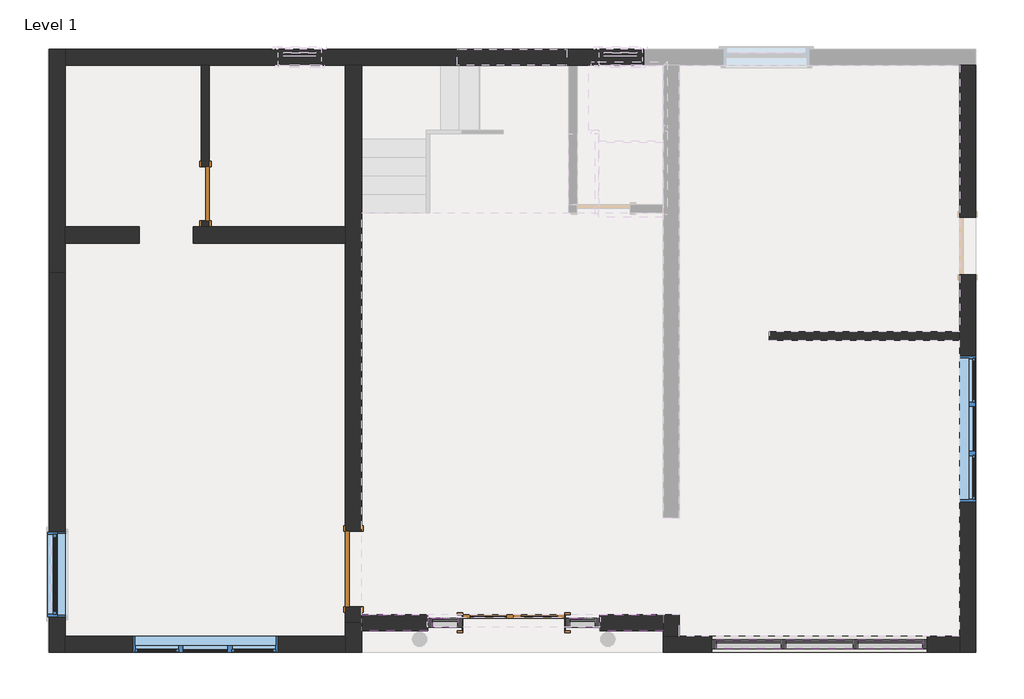
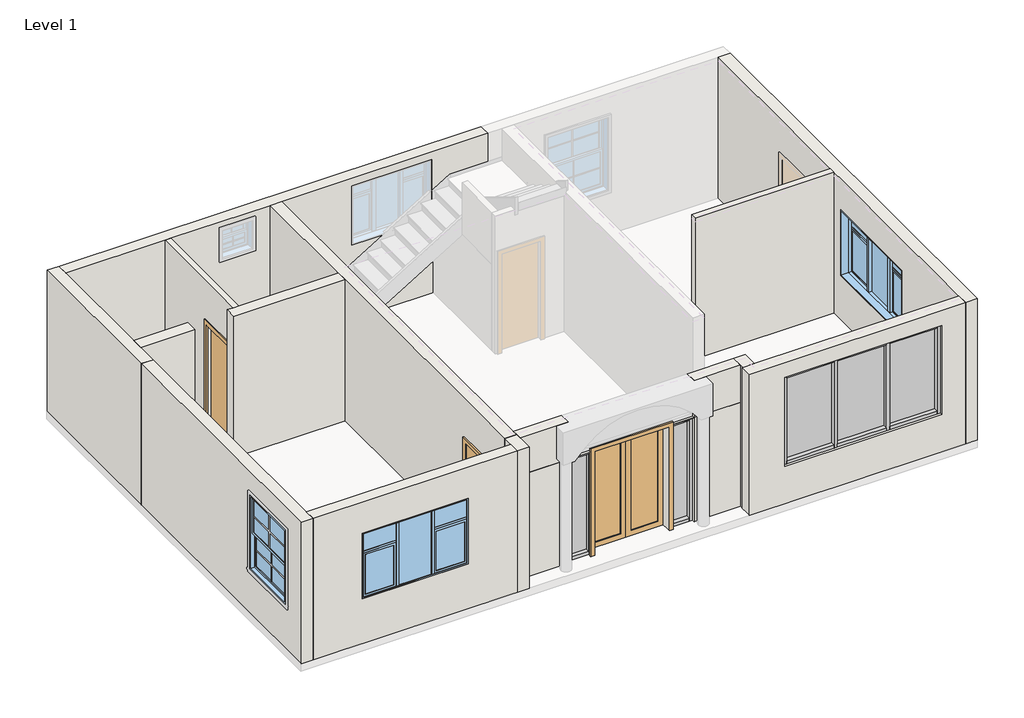
# One storey, part 1 of 2: 18 members, 16 walls, 5 plates, 3 doors, 3 windows.
"""IFC4 building model written with IfcOpenShell, lengths in millimetres."""

from ifc_helpers import new_model, si_unit, frame, origin, origin_with_axes, place, context, project, spatial, polyline, outline, extrude, faceted_brep, transform, mapped, element, save
from components import door_7b3e5dee, door_f6232a3f, door_d8f5dbb5, member_0417a2a7, member_3a4673bc, member_a7b41546, member_5da52246, member_04c9b82a, member_d60e8053, member_2fae0574, system_panel_glazed_7d1c9128, system_panel_glazed_4f997f60, system_panel_glazed_2247c2a6, system_panel_glazed_0f092676, window_casement_triple_side_transom_6_9_71562f8e, window_double_hung_3_11_b20011b0

model = new_model("IFC4")

# Units and contexts
model_context = context("Model", 3, world=origin())
ifc_project = project(units=[si_unit("LENGTHUNIT", "METRE", prefix="MILLI")], contexts=[model_context])

# Site, building, storey
site = spatial("IfcSite", under=ifc_project)
building = spatial("IfcBuilding", under=site)
storey = spatial("IfcBuildingStorey", under=building, Name="Level 1", Elevation=0.0)

# Doors
placement = place(None, origin())
door_shape = door_7b3e5dee(model_context)
element("IfcDoor", 1, ObjectType="Door-Double-Glass : 4'9\"x7'", at=placement, inside=storey, context=model_context, shape_type="MappedRepresentation", body=[
    mapped(door_shape, transform((-12852.2526022, 3914.7357665, 0.0), x_axis=(1.0, 0.0, 0.0), y_axis=(0.0, 1.0, 0.0), z_axis=(0.0, 0.0, 1.0))),
])
door_2_shape = door_f6232a3f(model_context)
element("IfcDoor", 2, ObjectType="Single-Flush : 3'6\"", at=placement, inside=storey, context=model_context, shape_type="MappedRepresentation", body=[
    mapped(door_2_shape, transform((-15119.0556236, 4679.1170165, 0.0), x_axis=(0.0, -1.0, 0.0), y_axis=(1.0, 0.0, 0.0), z_axis=(0.0, 0.0, 1.0))),
])
door_3_shape = door_d8f5dbb5(model_context)
element("IfcDoor", 3, ObjectType="Single-Flush : 30\" x 80\"", at=placement, inside=storey, context=model_context, shape_type="MappedRepresentation", body=[
    mapped(door_3_shape, transform((-17215.2240665, 9988.7207935, 0.0), x_axis=(0.0, -1.0, 0.0), y_axis=(1.0, 0.0, 0.0), z_axis=(0.0, 0.0, 1.0))),
])

# Members
member_shape = member_0417a2a7(model_context)
element("IfcMember", 4, ObjectType="Rectangular Mullion : 2.5\" x 5\" rectangular", at=placement, inside=storey, context=model_context, shape_type="MappedRepresentation", body=[
    mapped(member_shape, transform((-13645.6697078, 3917.1170165, 2128.2825), x_axis=(0.0, 0.0, 1.0), y_axis=(0.0, -1.0, 0.0), z_axis=(1.0, 0.0, 0.0))),
])
element("IfcMember", 5, ObjectType="Rectangular Mullion : 2.5\" x 5\" rectangular", at=placement, inside=storey, context=model_context, shape_type="MappedRepresentation", body=[
    mapped(member_shape, transform((-11697.1590017, 3917.1170165, 2130.0999183), x_axis=(0.0, 0.0, 1.0), y_axis=(0.0, -1.0, 0.0), z_axis=(1.0, 0.0, 0.0))),
])
element("IfcMember", 6, ObjectType="Rectangular Mullion : 2.5\" x 5\" rectangular", at=placement, inside=storey, context=model_context, shape_type="MappedRepresentation", body=[
    mapped(member_shape, transform((-14008.2736637, 3917.1170165, 0.0), x_axis=(0.0, 0.0, -1.0), y_axis=(0.0, -1.0, 0.0), z_axis=(-1.0, 0.0, 0.0))),
])
element("IfcMember", 7, ObjectType="Rectangular Mullion : 2.5\" x 5\" rectangular", at=placement, inside=storey, context=model_context, shape_type="MappedRepresentation", body=[
    mapped(member_shape, transform((-12059.7629576, 3917.1170165, 0.0), x_axis=(0.0, 0.0, -1.0), y_axis=(0.0, -1.0, 0.0), z_axis=(-1.0, 0.0, 0.0))),
])
member_2_shape = member_3a4673bc(model_context)
element("IfcMember", 8, ObjectType="Rectangular Mullion : 2.5\" x 5\" rectangular", at=placement, inside=storey, context=model_context, shape_type="MappedRepresentation", body=[
    mapped(member_2_shape, transform((-13582.1697078, 3917.1170165, 0.0), x_axis=(1.0, 0.0, 0.0), y_axis=(0.0, -1.0, 0.0), z_axis=(0.0, 0.0, -1.0))),
])
element("IfcMember", 9, ObjectType="Rectangular Mullion : 2.5\" x 5\" rectangular", at=placement, inside=storey, context=model_context, shape_type="MappedRepresentation", body=[
    mapped(member_2_shape, transform((-14071.7736637, 3917.1170165, 2128.2825), x_axis=(-1.0, 0.0, 0.0), y_axis=(0.0, -1.0, 0.0), z_axis=(0.0, 0.0, 1.0))),
])
member_3_shape = member_a7b41546(model_context)
element("IfcMember", 10, ObjectType="Rectangular Mullion : 2.5\" x 5\" rectangular", at=placement, inside=storey, context=model_context, shape_type="MappedRepresentation", body=[
    mapped(member_3_shape, transform((-11633.6590017, 3917.1170165, 0.0), x_axis=(1.0, 0.0, 0.0), y_axis=(0.0, -1.0, 0.0), z_axis=(0.0, 0.0, -1.0))),
])
element("IfcMember", 11, ObjectType="Rectangular Mullion : 2.5\" x 5\" rectangular", at=placement, inside=storey, context=model_context, shape_type="MappedRepresentation", body=[
    mapped(member_3_shape, transform((-12123.2629576, 3917.1170165, 2130.0999183), x_axis=(-1.0, 0.0, 0.0), y_axis=(0.0, -1.0, 0.0), z_axis=(0.0, 0.0, 1.0))),
])
member_4_shape = member_5da52246(model_context)
element("IfcMember", 12, ObjectType="Rectangular Mullion : 2.5\" x 5\" rectangular", at=placement, inside=storey, context=model_context, shape_type="MappedRepresentation", body=[
    mapped(member_4_shape, transform((-7064.7325804, 3612.4962903, 2590.8), x_axis=(0.0, 0.0, 1.0), y_axis=(0.0, -1.0, 0.0), z_axis=(1.0, 0.0, 0.0))),
])
element("IfcMember", 13, ObjectType="Rectangular Mullion : 2.5\" x 5\" rectangular", at=placement, inside=storey, context=model_context, shape_type="MappedRepresentation", body=[
    mapped(member_4_shape, transform((-9065.4060913, 3612.4962903, 2590.8), x_axis=(0.0, 0.0, 1.0), y_axis=(0.0, -1.0, 0.0), z_axis=(1.0, 0.0, 0.0))),
])
member_5_shape = member_04c9b82a(model_context)
element("IfcMember", 14, ObjectType="Rectangular Mullion : 2.5\" x 5\" rectangular", at=placement, inside=storey, context=model_context, shape_type="MappedRepresentation", body=[
    mapped(member_5_shape, transform((-8049.194336, 3612.4962903, 2590.8), x_axis=(0.0, 0.0, 1.0), y_axis=(0.0, -1.0, 0.0), z_axis=(1.0, 0.0, 0.0))),
])
element("IfcMember", 15, ObjectType="Rectangular Mullion : 2.5\" x 5\" rectangular", at=placement, inside=storey, context=model_context, shape_type="MappedRepresentation", body=[
    mapped(member_4_shape, transform((-9986.3678469, 3612.4962903, 762.0), x_axis=(0.0, 0.0, -1.0), y_axis=(0.0, -1.0, 0.0), z_axis=(-1.0, 0.0, 0.0))),
])
element("IfcMember", 16, ObjectType="Rectangular Mullion : 2.5\" x 5\" rectangular", at=placement, inside=storey, context=model_context, shape_type="MappedRepresentation", body=[
    mapped(member_4_shape, transform((-7985.694336, 3612.4962903, 762.0), x_axis=(0.0, 0.0, -1.0), y_axis=(0.0, -1.0, 0.0), z_axis=(-1.0, 0.0, 0.0))),
])
element("IfcMember", 17, ObjectType="Rectangular Mullion : 2.5\" x 5\" rectangular", at=placement, inside=storey, context=model_context, shape_type="MappedRepresentation", body=[
    mapped(member_5_shape, transform((-9001.9060913, 3612.4962903, 762.0), x_axis=(0.0, 0.0, -1.0), y_axis=(0.0, -1.0, 0.0), z_axis=(-1.0, 0.0, 0.0))),
])
member_6_shape = member_d60e8053(model_context)
element("IfcMember", 18, ObjectType="Rectangular Mullion : 2.5\" x 5\" rectangular", at=placement, inside=storey, context=model_context, shape_type="MappedRepresentation", body=[
    mapped(member_6_shape, transform((-9033.6560913, 3612.4962903, 762.0), x_axis=(1.0, 0.0, 0.0), y_axis=(0.0, -1.0, 0.0), z_axis=(0.0, 0.0, -1.0))),
])
element("IfcMember", 19, ObjectType="Rectangular Mullion : 2.5\" x 5\" rectangular", at=placement, inside=storey, context=model_context, shape_type="MappedRepresentation", body=[
    mapped(member_6_shape, transform((-8017.444336, 3612.4962903, 762.0), x_axis=(1.0, 0.0, 0.0), y_axis=(0.0, -1.0, 0.0), z_axis=(0.0, 0.0, -1.0))),
])
member_7_shape = member_2fae0574(model_context)
element("IfcMember", 20, ObjectType="Rectangular Mullion : 2.5\" x 5\" rectangular", at=placement, inside=storey, context=model_context, shape_type="MappedRepresentation", body=[
    mapped(member_7_shape, transform((-7001.2325804, 3612.4962903, 762.0), x_axis=(1.0, 0.0, 0.0), y_axis=(0.0, -1.0, 0.0), z_axis=(0.0, 0.0, -1.0))),
])
element("IfcMember", 21, ObjectType="Rectangular Mullion : 2.5\" x 5\" rectangular", at=placement, inside=storey, context=model_context, shape_type="MappedRepresentation", body=[
    mapped(member_7_shape, transform((-10049.8678469, 3612.4962903, 2590.8), x_axis=(-1.0, 0.0, 0.0), y_axis=(0.0, -1.0, 0.0), z_axis=(0.0, 0.0, 1.0))),
])

# Plates
system_panel_glazed_shape = system_panel_glazed_7d1c9128(model_context)
element("IfcPlate", 22, ObjectType="System Panel : Glazed", at=placement, inside=storey, context=model_context, shape_type="MappedRepresentation", body=[
    mapped(system_panel_glazed_shape, transform((-13826.9716857, 3917.1170165, 63.5), x_axis=(1.0, 0.0, 0.0), y_axis=(0.0, 1.0, 0.0), z_axis=(0.0, 0.0, 1.0))),
])
system_panel_glazed_2_shape = system_panel_glazed_4f997f60(model_context)
element("IfcPlate", 23, ObjectType="System Panel : Glazed", at=placement, inside=storey, context=model_context, shape_type="MappedRepresentation", body=[
    mapped(system_panel_glazed_2_shape, transform((-11878.4609796, 3917.1170165, 63.5), x_axis=(1.0, 0.0, 0.0), y_axis=(0.0, 1.0, 0.0), z_axis=(0.0, 0.0, 1.0))),
])
system_panel_glazed_3_shape = system_panel_glazed_2247c2a6(model_context)
element("IfcPlate", 24, ObjectType="System Panel : Glazed", at=placement, inside=storey, context=model_context, shape_type="MappedRepresentation", body=[
    mapped(system_panel_glazed_3_shape, transform((-9525.8869691, 3612.4962903, 825.5), x_axis=(1.0, 0.0, 0.0), y_axis=(0.0, 1.0, 0.0), z_axis=(0.0, 0.0, 1.0))),
])
element("IfcPlate", 25, ObjectType="System Panel : Glazed", at=placement, inside=storey, context=model_context, shape_type="MappedRepresentation", body=[
    mapped(system_panel_glazed_3_shape, transform((-7525.2134582, 3612.4962903, 825.5), x_axis=(1.0, 0.0, 0.0), y_axis=(0.0, 1.0, 0.0), z_axis=(0.0, 0.0, 1.0))),
])
system_panel_glazed_4_shape = system_panel_glazed_0f092676(model_context)
element("IfcPlate", 26, ObjectType="System Panel : Glazed", at=placement, inside=storey, context=model_context, shape_type="MappedRepresentation", body=[
    mapped(system_panel_glazed_4_shape, transform((-8525.5502137, 3612.4962903, 825.5), x_axis=(1.0, 0.0, 0.0), y_axis=(0.0, 1.0, 0.0), z_axis=(0.0, 0.0, 1.0))),
])

# Walls
element("IfcWall", 27, ObjectType="4.5\"", at=placement, inside=storey, context=model_context, shape_type="SweptSolid", body=[
    extrude(outline(polyline([(9607.7207935, 2032.0), (9607.7207935, 0.0), (9518.8207935, 0.0), (9518.8207935, 2895.6), (11804.9957578, 2895.6), (11804.9957578, 0.0), (10369.7207935, 0.0), (10369.7207935, 2032.0), (9607.7207935, 2032.0)])), frame((-17272.3740665, 0.0, 0.0), z_axis=(1.0, 0.0, 0.0), x_axis=(0.0, 1.0, 0.0)), (0.0, 0.0, 1.0), 114.3),
])
element("IfcWall", 28, ObjectType="4.5\"", at=placement, inside=storey, context=model_context, shape_type="SweptSolid", body=[
    extrude(outline(polyline([(-6545.326005, 7918.5333114), (-9237.1629596, 7918.5333114), (-9237.1629596, 8032.8333114), (-6545.326005, 8032.8333114), (-6545.326005, 7918.5333114)])), origin_with_axes(), (0.0, 0.0, 1.0), 2895.6),
])
element("IfcWall", 29, ObjectType="9\"", at=placement, inside=storey, context=model_context, shape_type="Brep", body=[
    faceted_brep([(-19425.7322207, 8869.9954766, 0.0), (-19425.7322207, 3498.1962903, 0.0), (-19425.7322207, 3498.1962903, 2895.6), (-19425.7322207, 8869.9954766, 2895.6), (-19425.7322207, 4006.1962903, 2438.4), (-19425.7322207, 4006.1962903, 914.4), (-19425.7322207, 5199.9962903, 914.4), (-19425.7322207, 5199.9962903, 2438.4), (-19197.1322207, 8869.9954766, 0.0), (-19197.1322207, 8869.9954766, 2895.6), (-19197.1322207, 3726.7962903, 2895.6), (-19197.1322207, 3498.1962903, 2895.6), (-19197.1322207, 3498.1962903, 0.0), (-19197.1322207, 3726.7962903, 0.0), (-19197.1322207, 4006.1962903, 2438.4), (-19197.1322207, 5199.9962903, 2438.4), (-19197.1322207, 5199.9962903, 914.4), (-19197.1322207, 4006.1962903, 914.4)], [[[0, 1, 2, 3], [4, 5, 6, 7]], [[8, 9, 10, 11, 12, 13], [14, 15, 16, 17]], [[1, 0, 8, 13, 12]], [[3, 2, 11, 10, 9]], [[0, 3, 9, 8]], [[2, 1, 12, 11]], [[5, 4, 14, 17]], [[6, 5, 17, 16]], [[7, 6, 16, 15]], [[4, 7, 15, 14]]]),
])
element("IfcWall", 30, ObjectType="9\"", at=placement, inside=storey, context=model_context, shape_type="Brep", body=[
    faceted_brep([(-19425.7322207, 12033.5957578, 0.0), (-19425.7322207, 8869.9954766, 0.0), (-19425.7322207, 8869.9954766, 2895.6), (-19425.7322207, 12033.5957578, 2895.6), (-19197.1322207, 12033.5957578, 0.0), (-19197.1322207, 12033.5957578, 2895.6), (-19197.1322207, 11804.9957578, 2895.6), (-19197.1322207, 9518.8207935, 2895.6), (-19197.1322207, 9290.2207935, 2895.6), (-19197.1322207, 8869.9954766, 2895.6), (-19197.1322207, 8869.9954766, 0.0), (-19197.1322207, 9290.2207935, 0.0), (-19197.1322207, 9518.8207935, 0.0), (-19197.1322207, 11804.9957578, 0.0)], [[[0, 1, 2, 3]], [[4, 5, 6, 7, 8, 9, 10, 11, 12, 13]], [[1, 0, 4, 13, 12, 11, 10]], [[2, 1, 10, 9]], [[3, 2, 9, 8, 7, 6, 5]], [[0, 3, 5, 4]]]),
])
element("IfcWall", 31, ObjectType="9\"", at=placement, inside=storey, context=model_context, shape_type="Brep", body=[
    faceted_brep([(-11009.5531945, 12033.5957578, 0.0), (-19197.1322207, 12033.5957578, 0.0), (-19197.1322207, 12033.5957578, 2895.6), (-11009.5531945, 12033.5957578, 2895.6), (-12102.8099332, 12033.5957578, 2743.2), (-13652.2099332, 12033.5957578, 2743.2), (-13652.2099332, 12033.5957578, 1524.0), (-12102.8099332, 12033.5957578, 1524.0), (-16185.8556236, 12033.5957578, 2743.2), (-16185.8556236, 12033.5957578, 2133.6), (-15576.2556236, 12033.5957578, 2133.6), (-15576.2556236, 12033.5957578, 2743.2), (-11644.5531945, 12033.5957578, 2133.6), (-11644.5531945, 12033.5957578, 1524.0), (-11034.9531945, 12033.5957578, 1524.0), (-11034.9531945, 12033.5957578, 2133.6), (-11009.5531945, 11804.9957578, 0.0), (-11009.5531945, 11804.9957578, 2895.6), (-15004.7556236, 11804.9957578, 2895.6), (-15233.3556236, 11804.9957578, 2895.6), (-17158.0740665, 11804.9957578, 2895.6), (-17272.3740665, 11804.9957578, 2895.6), (-19197.1322207, 11804.9957578, 2895.6), (-19197.1322207, 11804.9957578, 0.0), (-17272.3740665, 11804.9957578, 0.0), (-17158.0740665, 11804.9957578, 0.0), (-15233.3556236, 11804.9957578, 0.0), (-15004.7556236, 11804.9957578, 0.0), (-12071.0599332, 11804.9957578, 0.0), (-11956.7599332, 11804.9957578, 0.0), (-12102.8099332, 11804.9957578, 2743.2), (-12102.8099332, 11804.9957578, 1524.0), (-13652.2099332, 11804.9957578, 1524.0), (-13652.2099332, 11804.9957578, 2743.2), (-16185.8556236, 11804.9957578, 2743.2), (-15576.2556236, 11804.9957578, 2743.2), (-15576.2556236, 11804.9957578, 2133.6), (-16185.8556236, 11804.9957578, 2133.6), (-11644.5531945, 11804.9957578, 2133.6), (-11034.9531945, 11804.9957578, 2133.6), (-11034.9531945, 11804.9957578, 1524.0), (-11644.5531945, 11804.9957578, 1524.0)], [[[0, 1, 2, 3], [4, 5, 6, 7], [8, 9, 10, 11], [12, 13, 14, 15]], [[16, 17, 18, 19, 20, 21, 22, 23, 24, 25, 26, 27, 28, 29], [30, 31, 32, 33], [34, 35, 36, 37], [38, 39, 40, 41]], [[1, 0, 16, 29, 28, 27, 26, 25, 24, 23]], [[3, 2, 22, 21, 20, 19, 18, 17]], [[0, 3, 17, 16]], [[2, 1, 23, 22]], [[31, 30, 4, 7]], [[32, 31, 7, 6]], [[33, 32, 6, 5]], [[30, 33, 5, 4]], [[9, 8, 34, 37]], [[10, 9, 37, 36]], [[11, 10, 36, 35]], [[8, 11, 35, 34]], [[13, 12, 38, 41]], [[14, 13, 41, 40]], [[15, 14, 40, 39]], [[12, 15, 39, 38]]]),
])
element("IfcWall", 32, ObjectType="9\"", at=placement, inside=storey, context=model_context, shape_type="Brep", body=[
    faceted_brep([(-6315.3817031, 11804.9957578, 2895.6), (-6315.3817031, 3498.1962903, 2895.6), (-6315.3817031, 3498.1962903, 0.0), (-6315.3817031, 8845.8957578, 0.0), (-6315.3817031, 8845.8957578, 2133.6), (-6315.3817031, 9658.6957578, 2133.6), (-6315.3817031, 9658.6957578, 0.0), (-6315.3817031, 11804.9957578, 0.0), (-6315.3817031, 5632.7957578, 2260.6), (-6315.3817031, 7690.1957578, 2260.6), (-6315.3817031, 7690.1957578, 914.4), (-6315.3817031, 5632.7957578, 914.4), (-6543.9817031, 3498.1962903, 2895.6), (-6543.9817031, 3726.7962903, 2895.6), (-6543.9817031, 11804.9957578, 2895.6), (-6543.9817031, 11804.9957578, 0.0), (-6543.9817031, 9658.6957578, 0.0), (-6543.9817031, 9658.6957578, 2133.6), (-6543.9817031, 8845.8957578, 2133.6), (-6543.9817031, 8845.8957578, 0.0), (-6543.9817031, 3726.7962903, 0.0), (-6543.9817031, 3498.1962903, 0.0), (-6543.9817031, 5632.7957578, 2260.6), (-6543.9817031, 5632.7957578, 914.4), (-6543.9817031, 7690.1957578, 914.4), (-6543.9817031, 7690.1957578, 2260.6)], [[[0, 1, 2, 3, 4, 5, 6, 7], [8, 9, 10, 11]], [[12, 13, 14, 15, 16, 17, 18, 19, 20, 21], [22, 23, 24, 25]], [[15, 7, 6, 16]], [[2, 21, 20, 19, 3]], [[1, 0, 14, 13, 12]], [[0, 7, 15, 14]], [[2, 1, 12, 21]], [[4, 3, 19, 18]], [[5, 4, 18, 17]], [[6, 5, 17, 16]], [[23, 22, 8, 11]], [[24, 23, 11, 10]], [[25, 24, 10, 9]], [[22, 25, 9, 8]]]),
])
element("IfcWall", 33, ObjectType="9\"", at=placement, inside=storey, context=model_context, shape_type="Brep", body=[
    faceted_brep([(-10737.7026022, 3498.1962903, 0.0), (-6543.9817031, 3498.1962903, 0.0), (-6543.9817031, 3498.1962903, 2895.6), (-10737.7026022, 3498.1962903, 2895.6), (-10049.8678469, 3498.1962903, 762.0), (-10049.8678469, 3498.1962903, 2590.8), (-7001.2325804, 3498.1962903, 2590.8), (-7001.2325804, 3498.1962903, 762.0), (-6543.9817031, 3726.7962903, 0.0), (-10507.7583002, 3726.7962903, 0.0), (-10736.3583002, 3726.7962903, 0.0), (-10737.7026022, 3726.7962903, 0.0), (-10737.7026022, 3726.7962903, 2895.6), (-10736.3583002, 3726.7962903, 2895.6), (-10507.7583002, 3726.7962903, 2895.6), (-6543.9817031, 3726.7962903, 2895.6), (-10049.8678469, 3726.7962903, 2590.8), (-10049.8678469, 3726.7962903, 762.0), (-7001.2325804, 3726.7962903, 762.0), (-7001.2325804, 3726.7962903, 2590.8)], [[[0, 1, 2, 3], [4, 5, 6, 7]], [[8, 9, 10, 11, 12, 13, 14, 15], [16, 17, 18, 19]], [[1, 0, 11, 10, 9, 8]], [[3, 2, 15, 14, 13, 12]], [[0, 3, 12, 11]], [[2, 1, 8, 15]], [[4, 17, 16, 5]], [[6, 19, 18, 7]], [[17, 4, 7, 18]], [[19, 6, 5, 16]]]),
])
element("IfcWall", 34, ObjectType="9\"", at=placement, inside=storey, context=model_context, shape_type="SweptSolid", body=[
    extrude(outline(polyline([(-10507.7583002, 4031.4170165), (-10507.7583002, 3726.7962903), (-10736.3583002, 3726.7962903), (-10736.3583002, 4031.4170165), (-10507.7583002, 4031.4170165)])), origin_with_axes(), (0.0, 0.0, 1.0), 2895.6),
])
element("IfcWall", 35, ObjectType="9\"", at=placement, inside=storey, context=model_context, shape_type="Brep", body=[
    faceted_brep([(-10737.7026022, 4031.4170165, 2133.6), (-10737.7026022, 4031.4170165, 0.0), (-11633.6590017, 4031.4170165, 0.0), (-11633.6590017, 4031.4170165, 2130.0999183), (-12123.2629576, 4031.4170165, 2130.0999183), (-12123.2629576, 4031.4170165, 0.0), (-12128.3526022, 4031.4170165, 0.0), (-12128.3526022, 4031.4170165, 2133.6), (-11633.6590017, 4031.4170165, 2133.6), (-10737.7026022, 3802.8170165, 0.0), (-10737.7026022, 3802.8170165, 2133.6), (-11633.6590017, 3802.8170165, 2133.6), (-12128.3526022, 3802.8170165, 2133.6), (-12128.3526022, 3802.8170165, 0.0), (-12123.2629576, 3802.8170165, 0.0), (-12123.2629576, 3802.8170165, 2130.0999183), (-11633.6590017, 3802.8170165, 2130.0999183), (-11633.6590017, 3802.8170165, 0.0)], [[[0, 1, 2, 3, 4, 5, 6, 7, 8]], [[9, 10, 11, 12, 13, 14, 15, 16, 17]], [[1, 9, 17, 2]], [[13, 6, 5, 14]], [[10, 0, 8, 7, 12, 11]], [[1, 0, 10, 9]], [[7, 6, 13, 12]], [[4, 15, 14, 5]], [[16, 3, 2, 17]], [[3, 16, 15, 4]]]),
    faceted_brep([(-14071.7736637, 4031.4170165, 0.0), (-15004.7556236, 4031.4170165, 0.0), (-15004.7556236, 4031.4170165, 2133.6), (-14071.7736637, 4031.4170165, 2133.6), (-13576.1526022, 4031.4170165, 2133.6), (-13576.1526022, 4031.4170165, 0.0), (-13582.1697078, 4031.4170165, 0.0), (-13582.1697078, 4031.4170165, 2128.2825), (-14071.7736637, 4031.4170165, 2128.2825), (-15005.3951996, 3802.8170165, 2133.6), (-15005.3951996, 3802.8170165, 0.0), (-14071.7736637, 3802.8170165, 0.0), (-14071.7736637, 3802.8170165, 2128.2825), (-13582.1697078, 3802.8170165, 2128.2825), (-13582.1697078, 3802.8170165, 0.0), (-13576.1526022, 3802.8170165, 0.0), (-13576.1526022, 3802.8170165, 2133.6), (-14071.7736637, 3802.8170165, 2133.6), (-15005.3951996, 3917.1170165, 0.0), (-15004.7556236, 3917.1170165, 0.0), (-15004.7556236, 3917.1170165, 2133.6), (-15005.3951996, 3917.1170165, 2133.6)], [[[0, 1, 2, 3, 4, 5, 6, 7, 8]], [[9, 10, 11, 12, 13, 14, 15, 16, 17]], [[1, 0, 11, 10, 18, 19]], [[6, 5, 15, 14]], [[4, 3, 2, 20, 21, 9, 17, 16]], [[0, 8, 12, 11]], [[7, 6, 14, 13]], [[5, 4, 16, 15]], [[12, 8, 7, 13]], [[2, 1, 19, 20]], [[19, 18, 21, 20]], [[10, 9, 21, 18]]]),
])
element("IfcWall", 36, ObjectType="9\"", at=placement, inside=storey, context=model_context, shape_type="Brep", body=[
    faceted_brep([(-15233.3556236, 4145.7170165, 2032.0), (-15233.3556236, 4145.7170165, 0.0), (-15233.3556236, 3917.1170165, 0.0), (-15233.3556236, 3917.1170165, 2895.6), (-15233.3556236, 9290.2207935, 2895.6), (-15233.3556236, 9518.8207935, 2895.6), (-15233.3556236, 11804.9957578, 2895.6), (-15233.3556236, 11804.9957578, 0.0), (-15233.3556236, 9518.8207935, 0.0), (-15233.3556236, 9290.2207935, 0.0), (-15233.3556236, 5212.5170165, 0.0), (-15233.3556236, 5212.5170165, 2032.0), (-15004.7556236, 3917.1170165, 0.0), (-15004.7556236, 4031.4170165, 0.0), (-15004.7556236, 4145.7170165, 0.0), (-15004.7556236, 4145.7170165, 2032.0), (-15004.7556236, 5212.5170165, 2032.0), (-15004.7556236, 5212.5170165, 0.0), (-15004.7556236, 11804.9957578, 0.0), (-15004.7556236, 11804.9957578, 2895.6), (-15004.7556236, 4031.4170165, 2895.6), (-15004.7556236, 3917.1170165, 2895.6), (-15004.7556236, 3917.1170165, 2133.6), (-15005.3951996, 3917.1170165, 0.0), (-15005.3951996, 3917.1170165, 2895.6)], [[[0, 1, 2, 3, 4, 5, 6, 7, 8, 9, 10, 11]], [[12, 13, 14, 15, 16, 17, 18, 19, 20, 21, 22]], [[2, 1, 14, 13, 12, 23]], [[10, 9, 8, 7, 18, 17]], [[6, 5, 4, 3, 24, 21, 20, 19]], [[7, 6, 19, 18]], [[2, 23, 12, 22, 21, 24, 3]], [[15, 14, 1, 0]], [[16, 15, 0, 11]], [[17, 16, 11, 10]]]),
])
element("IfcWall", 37, ObjectType="9\"", at=placement, inside=storey, context=model_context, shape_type="Brep", body=[
    faceted_brep([(-15005.3951996, 3498.1962903, 0.0), (-15005.3951996, 3802.8170165, 0.0), (-15005.3951996, 3917.1170165, 0.0), (-15005.3951996, 3917.1170165, 2133.6), (-15005.3951996, 3917.1170165, 2895.6), (-15005.3951996, 3802.8170165, 2895.6), (-15005.3951996, 3498.1962903, 2895.6), (-15233.9951996, 3498.1962903, 0.0), (-15233.9951996, 3498.1962903, 2895.6), (-15233.9951996, 3726.7962903, 2895.6), (-15233.9951996, 3917.1170165, 2895.6), (-15233.9951996, 3917.1170165, 0.0), (-15233.9951996, 3726.7962903, 0.0), (-15233.3556236, 3917.1170165, 0.0), (-15233.3556236, 3917.1170165, 2895.6)], [[[0, 1, 2, 3, 4, 5, 6]], [[7, 8, 9, 10, 11, 12]], [[2, 1, 0, 7, 12, 11, 13]], [[6, 5, 4, 14, 10, 9, 8]], [[0, 6, 8, 7]], [[2, 13, 11, 10, 14, 4, 3]]]),
])
element("IfcWall", 38, ObjectType="9\"", at=placement, inside=storey, context=model_context, shape_type="SweptSolid", body=[
    extrude(outline(polyline([(0.0, -19197.1322207), (0.0, -15233.9951996), (2895.6, -15233.9951996), (2895.6, -19197.1322207), (0.0, -19197.1322207)]), holes=[polyline([(2260.6, -18244.2637102), (2260.6, -16186.8637102), (914.4, -16186.8637102), (914.4, -18244.2637102), (2260.6, -18244.2637102)])]), frame((0.0, 3498.1962903, 0.0), z_axis=(0.0, 1.0, 0.0), x_axis=(0.0, 0.0, 1.0)), (0.0, 0.0, 1.0), 228.6),
])
element("IfcWall", 39, ObjectType="9\"", at=placement, inside=storey, context=model_context, shape_type="SweptSolid", body=[
    extrude(outline(polyline([(-18149.1852461, 9290.2207935), (-19197.1322207, 9290.2207935), (-19197.1322207, 9518.8207935), (-18149.1852461, 9518.8207935), (-18149.1852461, 9290.2207935)])), origin_with_axes(), (0.0, 0.0, 1.0), 2895.6),
])
element("IfcWall", 40, ObjectType="9\"", at=placement, inside=storey, context=model_context, shape_type="Brep", body=[
    faceted_brep([(-17388.0183685, 9290.2207935, 0.0), (-15233.3556236, 9290.2207935, 0.0), (-15233.3556236, 9290.2207935, 2895.6), (-17388.0183685, 9290.2207935, 2895.6), (-17388.0183685, 9518.8207935, 0.0), (-17388.0183685, 9518.8207935, 2895.6), (-17272.3740665, 9518.8207935, 2895.6), (-17158.0740665, 9518.8207935, 2895.6), (-15233.3556236, 9518.8207935, 2895.6), (-15233.3556236, 9518.8207935, 0.0), (-17158.0740665, 9518.8207935, 0.0), (-17272.3740665, 9518.8207935, 0.0)], [[[0, 1, 2, 3]], [[4, 5, 6, 7, 8, 9, 10, 11]], [[1, 0, 4, 11, 10, 9]], [[3, 2, 8, 7, 6, 5]], [[0, 3, 5, 4]], [[2, 1, 9, 8]]]),
])
element("IfcWall", 41, ObjectType="9\"", at=placement, inside=storey, context=model_context, shape_type="SweptSolid", body=[
    extrude(outline(polyline([(-14071.7736637, 3802.8170165), (-15005.3951996, 3802.8170165), (-15005.3951996, 3917.1170165), (-15004.7556236, 3917.1170165), (-15004.7556236, 4031.4170165), (-14071.7736637, 4031.4170165), (-14071.7736637, 3802.8170165)])), frame((0.0, 0.0, 2133.6), z_axis=(0.0, 0.0, 1.0), x_axis=(1.0, 0.0, 0.0)), (0.0, 0.0, 1.0), 762.0),
])
element("IfcWall", 42, ObjectType="9\"", at=placement, inside=storey, context=model_context, shape_type="SweptSolid", body=[
    extrude(outline(polyline([(-10737.7026022, 3802.8170165), (-11633.6590017, 3802.8170165), (-11633.6590017, 4031.4170165), (-10737.7026022, 4031.4170165), (-10737.7026022, 3802.8170165)])), frame((0.0, 0.0, 2133.6), z_axis=(0.0, 0.0, 1.0), x_axis=(1.0, 0.0, 0.0)), (0.0, 0.0, 1.0), 762.0),
])

# Windows
window_casement_triple_side_transom_6_9_shape = window_casement_triple_side_transom_6_9_71562f8e(model_context)
element("IfcWindow", 43, ObjectType="Window-Casement-Triple-Side-Transom : 6'9", at=placement, inside=storey, context=model_context, shape_type="MappedRepresentation", body=[
    mapped(window_casement_triple_side_transom_6_9_shape, transform((-6429.6817031, 6661.4957578, 0.0), x_axis=(0.0, -1.0, 0.0), y_axis=(1.0, 0.0, 0.0), z_axis=(0.0, 0.0, 1.0))),
])
element("IfcWindow", 44, ObjectType="Window-Casement-Triple-Side-Transom : 6'9", at=placement, inside=storey, context=model_context, shape_type="MappedRepresentation", body=[
    mapped(window_casement_triple_side_transom_6_9_shape, transform((-17215.5637102, 3612.4962903, 0.0), x_axis=(-1.0, 0.0, 0.0), y_axis=(0.0, -1.0, 0.0), z_axis=(0.0, 0.0, 1.0))),
])
window_double_hung_3_11_shape = window_double_hung_3_11_b20011b0(model_context)
element("IfcWindow", 45, ObjectType="Window-Double-Hung : 3'11", at=placement, inside=storey, context=model_context, shape_type="MappedRepresentation", body=[
    mapped(window_double_hung_3_11_shape, transform((-19311.4322207, 4603.0962903, 0.0), x_axis=(0.0, 1.0, 0.0), y_axis=(-1.0, 0.0, 0.0), z_axis=(0.0, 0.0, 1.0))),
])

save(model, "model.ifc")

# Revit data of these elements
# Type "Door-Double-Glass : 4'9\"x7'"
#   Type Mark = "9"
#   Construction Type Id = "opn-d45"
#   Assembly Code = "C1020"
#   Analytic Construction = "Wood frame, double glass door "
#   W = 2' - 4 1/2"
#   Thickness = 0' - 2"
#   Thermal Resistance (R) = 1.8150 (h·ft²·°F)/BTU
#   Swing Angle [instance default] = 90.00°
#   Heat Transfer Coefficient (U) = 0.5510 BTU/(h·ft²·°F)
#   Height = 7' - 0"
#   Bottom Rail = 0' - 4"
#   Top Rail = 0' - 4"
#   Stiles = 0' - 4"
#   Trim Projection = 0' - 1"
#   Trim Width = 0' - 3"
#   Width = 4' - 9"
#   Define Thermal Properties by = 1
#   Glazing = Glass
#   Panel Material = Wood - Birch - Solid Stained Light Low Gloss
#   Trim Material = Paint - Sienna
#   Visual Light Transmittance = 0
#   Solar Heat Gain Coefficient = 0
#   Function = (empty or 0)
#   Wall Closure = (empty or 0)
# Type "Single-Flush : 3'6\""
#   Type Mark = "11"
#   Construction Type Id = "MDOOR"
#   Assembly Code = "C1020"
#   Analytic Construction = "Metal"
#   Thickness = 0' - 2"
#   Heat Transfer Coefficient (U) = 0.651978 BTU/(h·ft²·°F)
#   Height = 6' - 8"
#   Trim Projection Ext = 0' - 1"
#   Trim Projection Int = 0' - 1"
#   Trim Width = 0' - 3"
#   Width = 3' - 6"
#   Define Thermal Properties by = 1
#   Door Material = Door - Panel
#   Frame Material = Door - Frame
#   Visual Light Transmittance = 0
#   Solar Heat Gain Coefficient = 0
#   Function = (empty or 0)
#   Wall Closure = (empty or 0)
# Type "Single-Flush : 30\" x 80\""
#   Type Mark = "5"
#   Construction Type Id = "MDOOR"
#   Assembly Code = "C1020"
#   Analytic Construction = "Metal"
#   Thickness = 0' - 2"
#   Heat Transfer Coefficient (U) = 0.651978 BTU/(h·ft²·°F)
#   Height = 6' - 8"
#   Trim Projection Ext = 0' - 1"
#   Trim Projection Int = 0' - 1"
#   Trim Width = 0' - 3"
#   Width = 2' - 6"
#   Define Thermal Properties by = 1
#   Define Thermal Properties by = 1
#   Door Material = Door - Panel
#   Frame Material = Door - Frame
#   Visual Light Transmittance = 0
#   Solar Heat Gain Coefficient = 0
#   Function = (empty or 0)
#   Wall Closure = (empty or 0)
# Type "Rectangular Mullion : 2.5\" x 5\" rectangular"
#   built-in parameter 1007304 = 0.416667 (stored number, unit not read)
#   built-in parameter 1007301 = 0.104167 (stored number, unit not read)
#   built-in parameter 1007300 = 0.104167 (stored number, unit not read)
# Type "System Panel : Glazed"
#   Construction Type Id = "GSP4R"
#   Analytic Construction = "1/8 in Pilkington single glazing"
#   Visual Light Transmittance = 0.9
#   Solar Heat Gain Coefficient = 0.86
#   Heat Transfer Coefficient (U) = 1.18115 BTU/(h·ft²·°F)
#   Define Thermal Properties by = 1
# Type "4.5\""
#   Assembly Code = "B2010"
#   Layers, outside or top first: 0' - 4 1/2" no material (function 1)
# Type "9\""
#   Assembly Code = "B2010"
#   Layers, outside or top first: 0' - 9" no material (function 1)
# Type "Window-Casement-Triple-Side-Transom : 6'9"
#   Type Mark = "25"
#   Fire Rating = "0.5h"
#   Assembly Code = "B2020100"
#   Analytic Construction = "Double glazing - domestic"
#   Window Width = 2' - 3"
#   Window Inset [instance default] = 0' - 0 5/8"
#   Wall Thickness [instance default] = 0' - 6"
#   Visual Light Transmittance = 0.81
#   Transom Height Ratio = 0.3
#   Thermal Resistance (R) = 1.8146 (h·ft²·°F)/BTU
#   Solar Heat Gain Coefficient = 0.76
#   Rough Width = 6' - 9 1/2"
#   Rough Height = 4' - 5 1/2"
#   Open Window Height = 3' - 1.1"
#   Heat Transfer Coefficient (U) = 0.5511 BTU/(h·ft²·°F)
#   Height = 4' - 5"
#   Transom Height = 1' - 3.9"
#   Frame Gap 3 [instance default] = 0' - 1 83/128"
#   Frame Gap 2 [instance default] = 0' - 0 5/8"
#   Frame Gap 1 = 0' - 1 51/128"
#   Default Sill Height = 3' - 0"
#   Width = 6' - 9"
#   Frame Material = Metal - Aluminum
#   Glass Panel Material = Glass
#   Wall Closure = (empty or 0)
# Type "Window-Double-Hung : 3'11"
#   Type Mark = "21"
#   Fire Rating = "0.5h"
#   Construction Type Id = "DG-DR"
#   Assembly Code = "B2020100"
#   Analytic Construction = "Double glazing - domestic"
#   Wall Thickness [instance default] = 0' - 6"
#   Window Inset [instance default] = 0' - 0"
#   Visual Light Transmittance = 0.81
#   Thermal Resistance (R) = 1.8146 (h·ft²·°F)/BTU
#   Solar Heat Gain Coefficient = 0.76
#   Muntin Width = 3' - 5"
#   Muntin Height = 2' - 2 1/8"
#   Interior Wall Closure [instance default] = 0' - 1 1/2"
#   Rough Width = 3' - 11 1/2"
#   Rough Height = 5' - 0 1/2"
#   Frame Extension [instance default] = 0' - 1 1/4"
#   Exterior Wall Closure [instance default] = 0' - 0 1/2"
#   Extension Jamb [instance default] = 0' - 1 1/2"
#   Heat Transfer Coefficient (U) = 0.5511 BTU/(h·ft²·°F)
#   Height = 5' - 0"
#   Width = 3' - 11"
#   Top Muntin Visibility = yes
#   Indicator Visibility [instance default] = yes
#   Extension Jamb Visibility [instance default] = yes
#   Interior Trim Visibility [instance default] = yes
#   Exterior Trim Visibility [instance default] = yes
#   Define Thermal Properties by = 1
#   Bottom Muntin Visibility = yes
#   Muntin Pattern = Muntin Pattern_2x2 : Muntin Pattern_2x2
#   Interior Trim Material = Wood - Stained
#   Interior Trim = Trim-Window-Interior-Flat : Picture Frame
#   Exterior Trim Material = Clad - White
#   Exterior Trim = Trim-Window-Exterior-Flat : with Sill
#   Glass Panel Material = Glass
#   Exterior Frame Material = Clad - White
#   Interior Frame Material = Wood - Stained
#   Wall Closure = (empty or 0)
# Element 1 (IfcDoor, "Door-Double-Glass : 4'9\"x7'")
#   Swing Angle = 90.00°
#   Phase Created = New Construction
#   Materials on its faces: "Wood - Birch - Solid Stained Light Low Gloss", "Paint - Sienna", "Glass"
# Element 2 (IfcDoor, "Single-Flush : 3'6\"")
#   Phase Created = New Construction
#   Materials on its faces: "Door - Frame", "Door - Panel"
# Element 3 (IfcDoor, "Single-Flush : 30\" x 80\"")
#   Phase Created = New Construction
#   Materials on its faces: "Door - Frame", "Door - Panel"
# Elements 4, 5, 6, 7, 8, 9, 10, 11, 12, 13, 14, 15, 16, 17, 18, 19, 20, 21 (IfcMember, "Rectangular Mullion : 2.5\" x 5\" rectangular")
#   Phase Created = New Construction
#   Materials on its faces: "Aluminum"
# Elements 22, 23, 24, 25, 26 (IfcPlate, "System Panel : Glazed")
#   Phase Created = New Construction
#   Materials on its faces: "Glass"
# Elements 27, 28 (IfcWall, "4.5\"")
#   Top Offset = 0' - 0"
#   Base Offset = 0' - 0"
#   wall height = 9' - 6"
#   Phase Created = New Construction
#   Base Constraint = Level 1
#   Top Constraint = 1 slab level
#   Materials on its faces: "Default Wall"
# Elements 29, 30, 31, 32, 33, 34, 36, 37, 38, 39, 40 (IfcWall, "9\"")
#   Top Offset = 0' - 0"
#   Base Offset = 0' - 0"
#   wall height = 9' - 6"
#   Phase Created = New Construction
#   Base Constraint = Level 1
#   Top Constraint = 1 slab level
#   Materials on its faces: "Default Wall"
# Element 35 (IfcWall, "9\"")
#   Top Offset = -2' - 6"
#   Base Offset = 0' - 0"
#   wall height = 7' - 0"
#   Phase Created = New Construction
#   Base Constraint = Level 1
#   Top Constraint = 1 slab level
#   Materials on its faces: "Default Wall"
# Elements 41, 42 (IfcWall, "9\"")
#   built-in parameter 1001111 = 7' - 0"
#   Top Offset = 10' - 0"
#   Base Offset = 7' - 0"
#   Unconnected Height = 2' - 6"
#   wall height = 2' - 6"
#   Phase Created = New Construction
#   Base Constraint = Level 1
#   Materials on its faces: "Default Wall"
# Element 43 (IfcWindow, "Window-Casement-Triple-Side-Transom : 6'9")
#   Mark = "5"
#   Window Inset = 0' - 0 5/8"
#   Frame Gap 3 = 0' - 1 83/128"
#   Frame Gap 2 = 0' - 0 5/8"
#   Phase Created = New Construction
#   Materials on its faces: "Metal - Aluminum", "Glass"
# Element 44 (IfcWindow, "Window-Casement-Triple-Side-Transom : 6'9")
#   Mark = "14"
#   Window Inset = 0' - 0 5/8"
#   Frame Gap 3 = 0' - 1 83/128"
#   Frame Gap 2 = 0' - 0 5/8"
#   Phase Created = New Construction
#   Materials on its faces: "Metal - Aluminum", "Glass"
# Element 45 (IfcWindow, "Window-Double-Hung : 3'11")
#   Mark = "4"
#   Window Inset = 0' - 0"
#   Interior Wall Closure = 0' - 1 1/2"
#   Frame Extension = 0' - 1 1/4"
#   Exterior Wall Closure = 0' - 0 1/2"
#   Interior Trim Visibility = yes
#   Indicator Visibility = yes
#   Exterior Trim Visibility = yes
#   Phase Created = New Construction
#   Materials on its faces: "Wood - Stained", "Glass", "Clad - White"
# Materials
#   "Glass": class "Glass", colour RGB 154 182 205, transparency 0.85, Description = "Soda Lime Glass", Cost = 0
#   "Wood - Birch - Solid Stained Light Low Gloss": class "Wood", colour RGB 210 159 95, transparency 0, Cost = 0
#   "Paint - Sienna": colour RGB 118 70 51, transparency 0, Cost = 0
#   "Door - Panel": class "Wood", colour RGB 210 159 95, transparency 0, Cost = 0
#   "Door - Frame": colour RGB 118 70 51, transparency 0, Cost = 0
#   "Metal - Aluminum": class "Metal", colour RGB 247 247 247, transparency 0
#   "Wood - Stained": class "Wood", colour RGB 224 178 126, transparency 0, Cost = 0
#   "Clad - White": class "Wood", colour RGB 242 242 238, transparency 0, Cost = 0
#   "Aluminum": class "Metal", colour RGB 247 247 247, transparency 0, Description = "Aluminum 6061", Cost = 0
#   "Default Wall": colour RGB 128 128 128, transparency 0, Cost = 0
